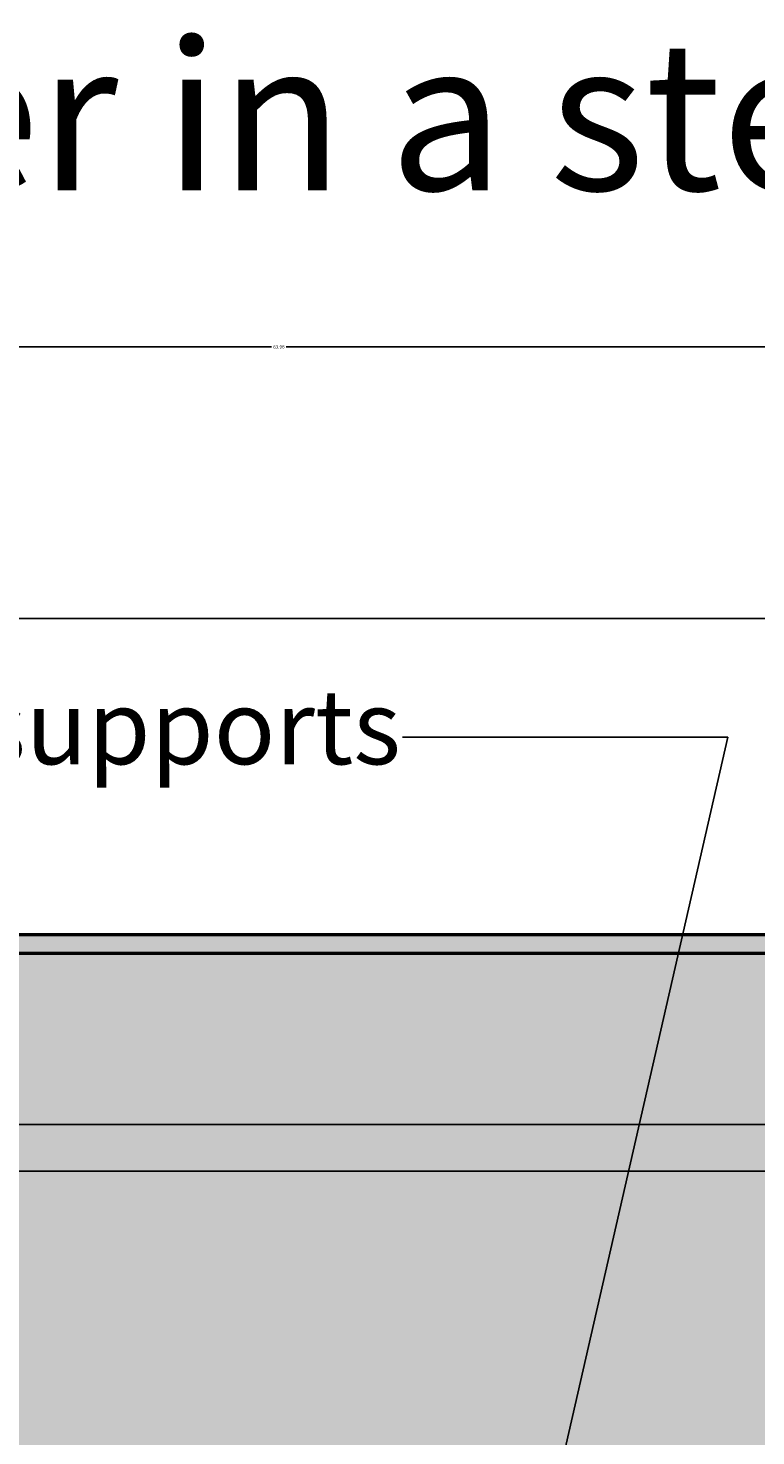
# Model space of a CAD drawing. Units: inches. Extents: x -12 to 334, y -10 to 186.
# Tile 62 of 77: x 145 to 184, y 111 to 186. Entities that reach past the tile are written whole.
import ezdxf
from ezdxf import colors
from ezdxf.entities.mleader import LeaderData, LeaderLine
from ezdxf.math import Vec2, Vec3

# ---------------------------------------------------------------- set-up
doc = ezdxf.new("R2010")
doc.units = ezdxf.units.IN
doc.header["$MEASUREMENT"] = 0
for name, color, linetype, lineweight in [('M-ANNO-TEXT', 3, 'Continuous', 25), ('M-DIMS', 2, 'Continuous', 18), ('M-EQPM', 7, 'Continuous', 50), ('M-EQPM-PATT', 8, 'Continuous', 18)]:
    doc.layers.add(name, color=color, linetype=linetype, lineweight=lineweight)
doc.styles.get("Standard").update_dxf_attribs({"font": 'arial.ttf'})
doc.dimstyles.get("Standard").update_dxf_attribs({"dimtxt": 0.18, "dimasz": 0.18, "dimexe": 0.18, "dimexo": 0.0625, "dimgap": 0.09, "dimtad": 0, "dimtih": 1, "dimtoh": 1, "dimdec": 4, "dimzin": 0, "dimdsep": 46, "dimtxsty": 'Standard', "dimcen": 0.09, "dimadec": 0, "dimazin": 0, "dimtfac": 1, "dimtdec": 4, "dimtofl": 0, "dimtmove": 0, "dimatfit": 3, "dimfxl": 1, "dimtolj": 1, "dimtzin": 0, "dimarcsym": 0})

# ---------------------------------------------------------------- blocks, each defined once
blk = doc.blocks.new('*D5')
at = {"layer": 'Defpoints', "color": 0, "transparency": 16777216}
for p in [(58.1, 127.708), (58.1, 125.208), (295.976, 125.208)]:
    blk.add_point(p, dxfattribs=at)
at = {"layer": 'M-DIMS', "color": 0, "lineweight": -2, "transparency": 16777216}
for p, q in [((58.163, 127.708), (296.156, 127.708)), ((295.976, 127.528), (295.976, 126.64)), ((295.976, 125.388), (295.976, 126.276)), ((58.163, 125.208), (296.156, 125.208))]:
    blk.add_line(p, q, dxfattribs=at)
at = {"layer": 'M-DIMS', "color": 0, "transparency": 16777216}
for points in [[(295.946, 127.528), (296.006, 127.528), (295.976, 127.708)], [(295.946, 125.388), (296.006, 125.388), (295.976, 125.208)]]:
    blk.add_solid(points, dxfattribs=at)
at = {"layer": 'M-DIMS', "color": 0, "transparency": 16777216, "insert": (295.976, 126.458), "char_height": 0.18, "attachment_point": 5}
blk.add_mtext('\\A1;2.5', dxfattribs=at)
blk = doc.blocks.new('*D18')
at = {"layer": 'Defpoints', "color": 0, "transparency": 16777216}
for p in [(190.342, 169.385), (190.342, 154.835), (126.379, 137.887)]:
    blk.add_point(p, dxfattribs=at)
at = {"layer": 'M-DIMS', "color": 0, "lineweight": -2, "transparency": 16777216}
for p, q in [((126.379, 137.95), (126.379, 169.565)), ((126.559, 169.385), (157.967, 169.385)), ((190.162, 169.385), (158.755, 169.385)), ((190.342, 154.897), (190.342, 169.565))]:
    blk.add_line(p, q, dxfattribs=at)
at = {"layer": 'M-DIMS', "color": 0, "transparency": 16777216}
for points in [[(126.559, 169.415), (126.559, 169.355), (126.379, 169.385)], [(190.162, 169.415), (190.162, 169.355), (190.342, 169.385)]]:
    blk.add_solid(points, dxfattribs=at)
at = {"layer": 'M-DIMS', "color": 0, "transparency": 16777216, "insert": (158.361, 169.385), "char_height": 0.18, "attachment_point": 5}
blk.add_mtext('\\A1;63.96', dxfattribs=at)
blk = doc.blocks.new('*D22')
at = {"layer": 'Defpoints', "color": 0, "transparency": 16777216}
for p in [(190.342, 154.835), (-11.174, 137.887), (195.342, 137.887)]:
    blk.add_point(p, dxfattribs=at)
at = {"layer": 'M-DIMS', "color": 0, "lineweight": -2, "transparency": 16777216}
for p, q in [((190.28, 154.835), (-11.354, 154.835)), ((-11.174, 154.655), (-11.174, 146.543)), ((-11.174, 138.067), (-11.174, 146.179)), ((195.28, 137.887), (-11.354, 137.887))]:
    blk.add_line(p, q, dxfattribs=at)
at = {"layer": 'M-DIMS', "color": 0, "transparency": 16777216}
for points in [[(-11.204, 154.655), (-11.144, 154.655), (-11.174, 154.835)], [(-11.204, 138.067), (-11.144, 138.067), (-11.174, 137.887)]]:
    blk.add_solid(points, dxfattribs=at)
at = {"layer": 'M-DIMS', "color": 0, "transparency": 16777216, "insert": (-11.174, 146.361), "char_height": 0.18, "attachment_point": 5}
blk.add_mtext('\\A1;16.947', dxfattribs=at)

msp = doc.modelspace()

# ---------------------------------------------------------------- hatches: boundary and pattern name
at = {"layer": 'M-EQPM-PATT', "transparency": 33554556}
h = msp.add_hatch(color=256, dxfattribs=at)
h.set_gradient(color1=(248, 206, 179), color2=(248, 206, 179), tint=1)
h.paths.add_polyline_path([(179.7818, 136.8871), (126.9567, 136.8871), (106.1771, 100.8958), (171.5458, 100.8958)])
h.paths.add_polyline_path([(268.3808, 136.9435), (214.0166, 136.9435), (214.0166, 154.8345), (196.3421, 154.8345), (196.3421, 136.8871), (179.7818, 136.8871), (171.5458, 100.8958), (231.7758, 100.8958, -0.4142136), (251.9801, 80.6915), (279.7263, 80.6915, 0.1631825)])
at = {"layer": 'M-EQPM-PATT'}
h = msp.add_hatch(color=256, dxfattribs=at)
h.set_gradient(color1=(99, 100, 102), color2=(99, 100, 102), tint=1)
h.paths.add_polyline_path([(126.9567, 136.8871), (179.7818, 136.8871), (180.0106, 137.8871), (126.3793, 137.8871), (106.1771, 102.8958), (86.8879, 102.8958), (86.8879, 109.0583), (84.7229, 109.0583), (84.7229, 100.8958), (106.1771, 100.8958)])
h.paths.add_polyline_path([(196.3421, 152.8345), (195.3421, 152.8345), (195.3421, 137.8871), (180.0106, 137.8871), (179.7818, 136.8871), (196.3421, 136.8871)])
h.paths.add_polyline_path([(215.0166, 152.8345), (214.0166, 152.8345), (214.0166, 136.9435), (268.3808, 136.9435, -0.2673785), (268.3808, 46.8541), (249.3759, 46.8541), (249.8485, 45.8541), (269.3808, 45.8541, 0.2615891), (269.3808, 137.9435), (215.0166, 137.9435)])

# ---------------------------------------------------------------- linework, layer by layer
at = {"layer": 'M-EQPM'}
for points in [[(106.1771, 100.8958), (126.9567, 136.8871), (196.3421, 136.8871), (196.3421, 154.8345)], [(106.1771, 102.8958), (126.3793, 137.8871), (195.3421, 137.8871), (195.3421, 152.8345)]]:
    msp.add_lwpolyline(points, dxfattribs=at)

# ---------------------------------------------------------------- texts
at = {"layer": 'M-ANNO-TEXT', "insert": (70.1252, 185.7805), "char_height": 8, "attachment_point": 1}
msp.add_mtext_dynamic_manual_height_columns('Heat exchanger in a steam boiler', width=205.597506, gutter_width=1, heights=[0], dxfattribs=at)

# ---------------------------------------------------------------- dimensions: what is measured, and where the dimension line sits
at = {"layer": 'M-DIMS'}
dim = msp.add_linear_dim(base=(190.3421, 169.3845), p1=(126.3793, 137.8871), p2=(190.3421, 154.8345), dimstyle='Standard', override={"dimdec": 2, "dimlfac": 1, "dimrnd": 0, "dimzin": 0, "dimdsep": 46, "dimlunit": 2}, dxfattribs=at)
dim.commit()
dim.dimension.update_dxf_attribs({"geometry": '*D18', "text_midpoint": (158.3607, 169.3845)})
for base, p1, p2, override, picture, middle in [((-11.1736, 137.8871), (190.3421, 154.8345), (195.3421, 137.8871), {"dimdec": 3, "dimlfac": 1, "dimrnd": 0, "dimzin": 0, "dimdsep": 46, "dimlunit": 2}, '*D22', (-11.1735, 146.3608)), ((295.9756, 125.2078), (58.1002, 127.7078), (58.1002, 125.2078), {"dimdec": 1, "dimlfac": 1, "dimrnd": 0, "dimzin": 0, "dimdsep": 46, "dimlunit": 2}, '*D5', (295.9756, 126.4578))]:
    dim = msp.add_linear_dim(base=base, p1=p1, p2=p2, angle=90, dimstyle='Standard', override=override, dxfattribs=at)
    dim.commit()
    dim.dimension.update_dxf_attribs({"geometry": picture, "text_midpoint": middle})

# ---------------------------------------------------------------- leaders
at = {"layer": 'M-ANNO-TEXT'}
ml = msp.add_multileader_mtext('Standard', dxfattribs=at)
ml.set_content('Tube supports', color=256)
ml.set_leader_properties()
ml.build(insert=Vec2(0, 0))
ml.multileader.update_dxf_attribs({"dogleg_length": 0.36, "arrow_head_size": 0.7})
ctx = ml.context
ctx.base_point, ctx.arrow_head_size, ctx.landing_gap_size, ctx.plane_origin = Vec3(129.4363, 148.4609), 0.7, 0.09, Vec3(117.375, 151.6517)
ctx.text_align_type = 2
notes = []
notes.append((ctx, [(1, (1, 1, 0), (182.4302, 148.4609), (-1, 0), 17.4388, [(0, [(170.9079, 98.1081)], 0, [])])]))
ctx.mtext.insert, ctx.mtext.alignment, ctx.mtext.flow_direction = Vec3(164.9015, 151.0162), 3, 5
for ctx, leaders in notes:
    for number, flags, end, landing, length, lines in leaders:
        leader = LeaderData()
        leader.index, (leader.has_last_leader_line, leader.has_dogleg_vector, leader.attachment_direction) = number, flags
        leader.last_leader_point, leader.dogleg_vector, leader.dogleg_length = Vec3(end), Vec3(landing), length
        for number, points, colour, breaks in lines:
            line = LeaderLine()
            line.index, line.vertices, line.color, line.breaks = number, Vec3.list(points), colors.encode_raw_color(colour), breaks
            leader.lines.append(line)
        ctx.leaders.append(leader)

doc.saveas('drawing.dxf')
